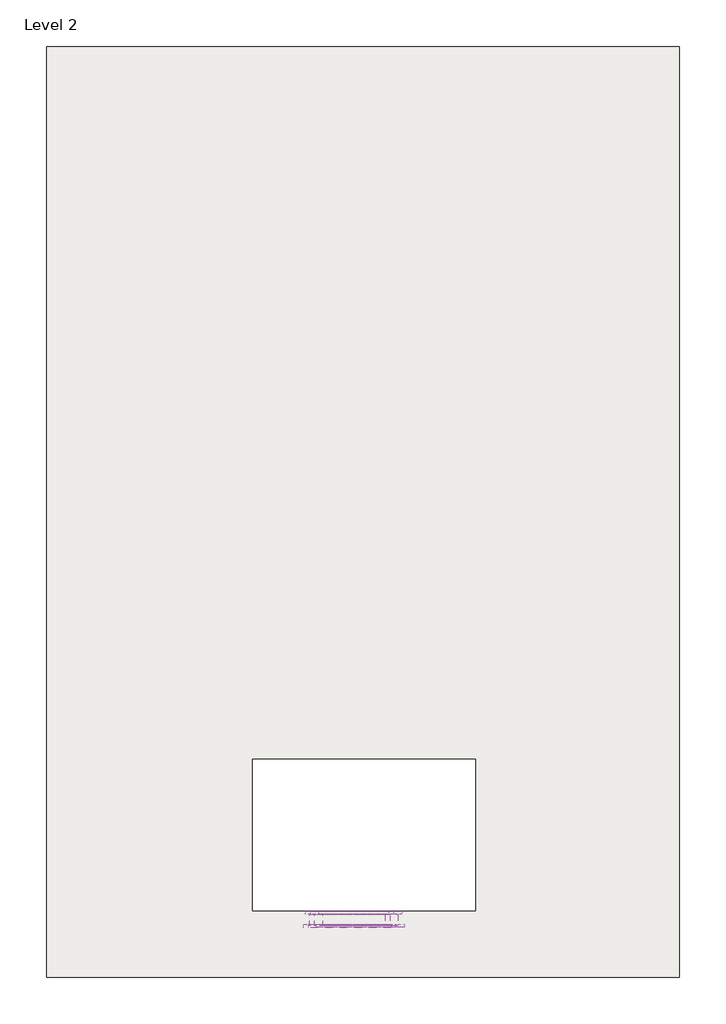
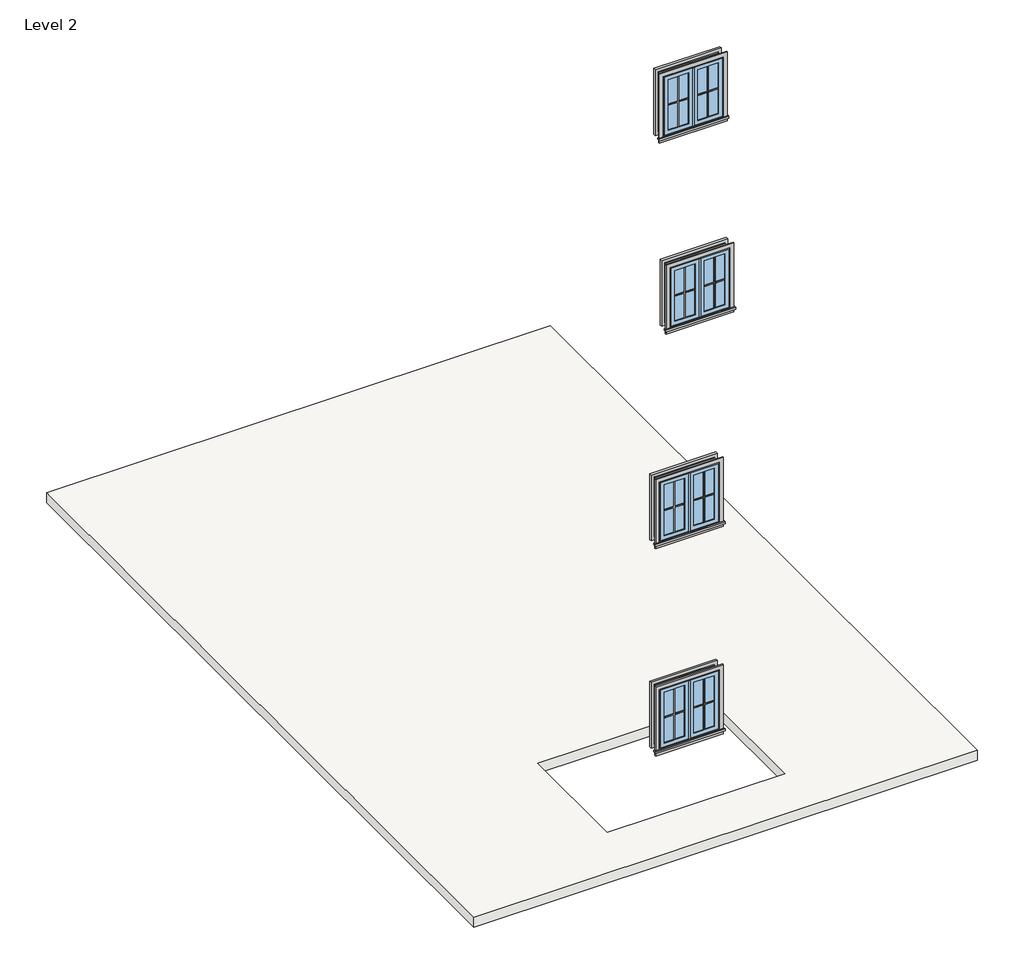
# One storey, incomplete: 16 proxies, 4 windows, 1 roof.
"""IFC4 building model written with IfcOpenShell, lengths in millimetres."""

from ifc_helpers import new_model, si_unit, frame, origin, place, context, project, spatial, polyline, outline, extrude, transform, mapped, element, save
from components import muntin_pattern_2x2_muntin_pattern_2x2_b3fe6957, muntin_pattern_2x2_muntin_pattern_2x2_3e0ecaf2, trim_window_exterior_flat_with_sill_41619996, trim_window_interior_flat_picture_frame_51c85655, window_a598f463

model = new_model("IFC4")

# Units and contexts
model_context = context("Model", 3, world=origin())
ifc_project = project(units=[si_unit("LENGTHUNIT", "METRE", prefix="MILLI")], contexts=[model_context])

# Site, building, storey
site = spatial("IfcSite", under=ifc_project)
building = spatial("IfcBuilding", under=site)
storey = spatial("IfcBuildingStorey", under=building, Name="Level 2", Elevation=3048.0)

# Proxies
placement = place(None, origin())
muntin_pattern_2x2_muntin_pattern_2x2_shape = muntin_pattern_2x2_muntin_pattern_2x2_b3fe6957(model_context)
element("IfcBuildingElementProxy", 1, Name="Muntin Pattern_2x2 : Muntin Pattern_2x2", ObjectType="Muntin Pattern_2x2 : Muntin Pattern_2x2", at=placement, inside=storey, context=model_context, shape_type="MappedRepresentation", body=[
    mapped(muntin_pattern_2x2_muntin_pattern_2x2_shape, transform((-1374.3964614, -4419.8859248, 4410.0195631), x_axis=(-1.0, 0.0, 0.0), y_axis=(0.0, -1.0, 0.0), z_axis=(0.0, 0.0, 1.0))),
])
element("IfcBuildingElementProxy", 2, Name="Muntin Pattern_2x2 : Muntin Pattern_2x2", ObjectType="Muntin Pattern_2x2 : Muntin Pattern_2x2", at=placement, inside=storey, context=model_context, shape_type="MappedRepresentation", body=[
    mapped(muntin_pattern_2x2_muntin_pattern_2x2_shape, transform((-1374.3964614, -4419.8859248, 7567.8197748), x_axis=(-1.0, 0.0, 0.0), y_axis=(0.0, -1.0, 0.0), z_axis=(0.0, 0.0, 1.0))),
])
element("IfcBuildingElementProxy", 3, Name="Muntin Pattern_2x2 : Muntin Pattern_2x2", ObjectType="Muntin Pattern_2x2 : Muntin Pattern_2x2", at=placement, inside=storey, context=model_context, shape_type="MappedRepresentation", body=[
    mapped(muntin_pattern_2x2_muntin_pattern_2x2_shape, transform((-1221.9964614, -4419.8859248, 10781.9890194), x_axis=(-1.0, 0.0, 0.0), y_axis=(0.0, -1.0, 0.0), z_axis=(0.0, 0.0, 1.0))),
])
element("IfcBuildingElementProxy", 4, Name="Muntin Pattern_2x2 : Muntin Pattern_2x2", ObjectType="Muntin Pattern_2x2 : Muntin Pattern_2x2", at=placement, inside=storey, context=model_context, shape_type="MappedRepresentation", body=[
    mapped(muntin_pattern_2x2_muntin_pattern_2x2_shape, transform((-1317.2464614, -4419.8859248, 13724.8067311), x_axis=(-1.0, 0.0, 0.0), y_axis=(0.0, -1.0, 0.0), z_axis=(0.0, 0.0, 1.0))),
])
muntin_pattern_2x2_muntin_pattern_2x2_2_shape = muntin_pattern_2x2_muntin_pattern_2x2_3e0ecaf2(model_context)
element("IfcBuildingElementProxy", 5, Name="Muntin Pattern_2x2 : Muntin Pattern_2x2", ObjectType="Muntin Pattern_2x2 : Muntin Pattern_2x2", at=placement, inside=storey, context=model_context, shape_type="MappedRepresentation", body=[
    mapped(muntin_pattern_2x2_muntin_pattern_2x2_2_shape, transform((-1803.0214614, -4419.8859248, 4410.0195631), x_axis=(1.0, 0.0, 0.0), y_axis=(0.0, 1.0, 0.0), z_axis=(0.0, 0.0, 1.0))),
])
element("IfcBuildingElementProxy", 6, Name="Muntin Pattern_2x2 : Muntin Pattern_2x2", ObjectType="Muntin Pattern_2x2 : Muntin Pattern_2x2", at=placement, inside=storey, context=model_context, shape_type="MappedRepresentation", body=[
    mapped(muntin_pattern_2x2_muntin_pattern_2x2_2_shape, transform((-1803.0214614, -4419.8859248, 7567.8197748), x_axis=(1.0, 0.0, 0.0), y_axis=(0.0, 1.0, 0.0), z_axis=(0.0, 0.0, 1.0))),
])
element("IfcBuildingElementProxy", 7, Name="Muntin Pattern_2x2 : Muntin Pattern_2x2", ObjectType="Muntin Pattern_2x2 : Muntin Pattern_2x2", at=placement, inside=storey, context=model_context, shape_type="MappedRepresentation", body=[
    mapped(muntin_pattern_2x2_muntin_pattern_2x2_2_shape, transform((-1650.6214614, -4419.8859248, 10781.9890194), x_axis=(1.0, 0.0, 0.0), y_axis=(0.0, 1.0, 0.0), z_axis=(0.0, 0.0, 1.0))),
])
element("IfcBuildingElementProxy", 8, Name="Muntin Pattern_2x2 : Muntin Pattern_2x2", ObjectType="Muntin Pattern_2x2 : Muntin Pattern_2x2", at=placement, inside=storey, context=model_context, shape_type="MappedRepresentation", body=[
    mapped(muntin_pattern_2x2_muntin_pattern_2x2_2_shape, transform((-1745.8714614, -4419.8859248, 13724.8067311), x_axis=(1.0, 0.0, 0.0), y_axis=(0.0, 1.0, 0.0), z_axis=(0.0, 0.0, 1.0))),
])
trim_window_exterior_flat_with_sill_shape = trim_window_exterior_flat_with_sill_41619996(model_context)
element("IfcBuildingElementProxy", 9, Name="Trim-Window-Exterior-Flat : with Sill", ObjectType="Trim-Window-Exterior-Flat : with Sill", at=placement, inside=storey, context=model_context, shape_type="MappedRepresentation", body=[
    mapped(trim_window_exterior_flat_with_sill_shape, transform((-1588.7089614, -4429.4109248, 5254.5695631), x_axis=(1.0, 0.0, 0.0), y_axis=(0.0, 0.0, 1.0), z_axis=(0.0, -1.0, 0.0))),
])
element("IfcBuildingElementProxy", 10, Name="Trim-Window-Exterior-Flat : with Sill", ObjectType="Trim-Window-Exterior-Flat : with Sill", at=placement, inside=storey, context=model_context, shape_type="MappedRepresentation", body=[
    mapped(trim_window_exterior_flat_with_sill_shape, transform((-1588.7089614, -4429.4109248, 8412.3697748), x_axis=(1.0, 0.0, 0.0), y_axis=(0.0, 0.0, 1.0), z_axis=(0.0, -1.0, 0.0))),
])
element("IfcBuildingElementProxy", 11, Name="Trim-Window-Exterior-Flat : with Sill", ObjectType="Trim-Window-Exterior-Flat : with Sill", at=placement, inside=storey, context=model_context, shape_type="MappedRepresentation", body=[
    mapped(trim_window_exterior_flat_with_sill_shape, transform((-1436.3089614, -4429.4109248, 11626.5390194), x_axis=(1.0, 0.0, 0.0), y_axis=(0.0, 0.0, 1.0), z_axis=(0.0, -1.0, 0.0))),
])
element("IfcBuildingElementProxy", 12, Name="Trim-Window-Exterior-Flat : with Sill", ObjectType="Trim-Window-Exterior-Flat : with Sill", at=placement, inside=storey, context=model_context, shape_type="MappedRepresentation", body=[
    mapped(trim_window_exterior_flat_with_sill_shape, transform((-1531.5589614, -4429.4109248, 14569.3567311), x_axis=(1.0, 0.0, 0.0), y_axis=(0.0, 0.0, 1.0), z_axis=(0.0, -1.0, 0.0))),
])
trim_window_interior_flat_picture_frame_shape = trim_window_interior_flat_picture_frame_51c85655(model_context)
element("IfcBuildingElementProxy", 13, Name="Trim-Window-Interior-Flat : Picture Frame", ObjectType="Trim-Window-Interior-Flat : Picture Frame", at=placement, inside=storey, context=model_context, shape_type="MappedRepresentation", body=[
    mapped(trim_window_interior_flat_picture_frame_shape, transform((-1588.7089614, -4315.1109248, 5254.5695631), x_axis=(-1.0, 0.0, 0.0), y_axis=(0.0, 0.0, 1.0), z_axis=(0.0, 1.0, 0.0))),
])
element("IfcBuildingElementProxy", 14, Name="Trim-Window-Interior-Flat : Picture Frame", ObjectType="Trim-Window-Interior-Flat : Picture Frame", at=placement, inside=storey, context=model_context, shape_type="MappedRepresentation", body=[
    mapped(trim_window_interior_flat_picture_frame_shape, transform((-1588.7089614, -4315.1109248, 8412.3697748), x_axis=(-1.0, 0.0, 0.0), y_axis=(0.0, 0.0, 1.0), z_axis=(0.0, 1.0, 0.0))),
])
element("IfcBuildingElementProxy", 15, Name="Trim-Window-Interior-Flat : Picture Frame", ObjectType="Trim-Window-Interior-Flat : Picture Frame", at=placement, inside=storey, context=model_context, shape_type="MappedRepresentation", body=[
    mapped(trim_window_interior_flat_picture_frame_shape, transform((-1436.3089614, -4315.1109248, 11626.5390194), x_axis=(-1.0, 0.0, 0.0), y_axis=(0.0, 0.0, 1.0), z_axis=(0.0, 1.0, 0.0))),
])
element("IfcBuildingElementProxy", 16, Name="Trim-Window-Interior-Flat : Picture Frame", ObjectType="Trim-Window-Interior-Flat : Picture Frame", at=placement, inside=storey, context=model_context, shape_type="MappedRepresentation", body=[
    mapped(trim_window_interior_flat_picture_frame_shape, transform((-1531.5589614, -4315.1109248, 14569.3567311), x_axis=(-1.0, 0.0, 0.0), y_axis=(0.0, 0.0, 1.0), z_axis=(0.0, 1.0, 0.0))),
])

# Roof
element("IfcRoof", 17, ObjectType="Generic - 12\"", at=placement, inside=storey, context=model_context, shape_type="SweptSolid", body=[
    extrude(outline(polyline([(2221.2910386, -5039.0109248), (-5036.7589614, -5039.0109248), (-5036.7589614, 5628.9890752), (2221.2910386, 5628.9890752), (2221.2910386, -5039.0109248)]), holes=[polyline([(-116.1777511, -2539.253904), (-2673.8853157, -2539.253904), (-2673.8853157, -4276.2080688), (-116.1777511, -4276.2080688), (-116.1777511, -2539.253904)])]), frame((0.0, 0.0, 3048.0), z_axis=(0.0, 0.0, 1.0), x_axis=(1.0, 0.0, 0.0)), (0.0, 0.0, 1.0), 152.4),
])

# Windows
window_shape = window_a598f463(model_context)
element("IfcWindow", 18, ObjectType="Window-Casement-Double : 34\" x 36\"", at=placement, inside=storey, context=model_context, shape_type="MappedRepresentation", body=[
    mapped(window_shape, transform((-1588.7089614, -4372.2609248, 3425.7695631), x_axis=(-1.0, 0.0, 0.0), y_axis=(0.0, -1.0, 0.0), z_axis=(0.0, 0.0, 1.0))),
])
element("IfcWindow", 19, ObjectType="Window-Casement-Double : 34\" x 36\"", at=placement, inside=storey, context=model_context, shape_type="MappedRepresentation", body=[
    mapped(window_shape, transform((-1588.7089614, -4372.2609248, 6583.5697748), x_axis=(-1.0, 0.0, 0.0), y_axis=(0.0, -1.0, 0.0), z_axis=(0.0, 0.0, 1.0))),
])
element("IfcWindow", 20, ObjectType="Window-Casement-Double : 34\" x 36\"", at=placement, inside=storey, context=model_context, shape_type="MappedRepresentation", body=[
    mapped(window_shape, transform((-1436.3089614, -4372.2609248, 9797.7390194), x_axis=(-1.0, 0.0, 0.0), y_axis=(0.0, -1.0, 0.0), z_axis=(0.0, 0.0, 1.0))),
])
element("IfcWindow", 21, ObjectType="Window-Casement-Double : 34\" x 36\"", at=placement, inside=storey, context=model_context, shape_type="MappedRepresentation", body=[
    mapped(window_shape, transform((-1531.5589614, -4372.2609248, 12740.5567311), x_axis=(-1.0, 0.0, 0.0), y_axis=(0.0, -1.0, 0.0), z_axis=(0.0, 0.0, 1.0))),
])

save(model, "model.ifc")

# Revit data of these elements
# Type "Muntin Pattern_2x2 : Muntin Pattern_2x2"
#   Width [instance default] = 4' - 0"
#   Thickness = 0' - 0 1/2"
#   Height [instance default] = 4' - 0"
#   Distance = 0' - 0 3/4"
#   Interior Material [instance default] = none
#   Exterior Material [instance default] = none
#   Default Elevation = 0
# Type "Trim-Window-Exterior-Flat : with Sill"
#   Trim Width = 0' - 2 1/4"
#   Trim Thickness_Picture Frame = 0' - 1 1/4"
#   Trim Thickness_with Sill = 0' - 0 3/4"
#   Sill Thickness = 0' - 1 1/4"
#   Opening Width [instance default] = 2' - 0"
#   Opening Height [instance default] = 3' - 0"
#   Default Elevation = 4' - 0"
#   Sill = yes
#   Picture Frame = no
#   Trim Material [instance default] = none
# Type "Trim-Window-Interior-Flat : Picture Frame"
#   Trim Thickness_Picture Frame = 0' - 1 1/4"
#   Trim Width = 0' - 2 1/4"
#   Trim Thickness_with Sill = 0' - 0 3/4"
#   Sill Thickness = 0' - 1 1/4"
#   Opening Width [instance default] = 2' - 0"
#   Opening Height [instance default] = 3' - 0"
#   Default Elevation = 4' - 0"
#   Sill = no
#   Picture Frame = yes
#   Trim Material [instance default] = none
# Type "Generic - 12\""
#   Assembly Code = "B1020"
#   Layers, outside or top first: 0' - 6" no material (function 1)
# Type "Window-Casement-Double : 34\" x 36\""
#   Type Mark = "14"
#   Fire Rating = "0.5h"
#   Assembly Code = "B2020100"
#   Analytic Construction = "Double glazing - domestic"
#   Frame Extension [instance default] = 0' - 0 1/4"
#   Window Inset [instance default] = 0' - 0"
#   Wall Thickness [instance default] = 0' - 6"
#   Interior Wall Closure [instance default] = 0' - 2 1/4"
#   Half Width = 1' - 5"
#   Visual Light Transmittance = 0.81
#   Thermal Resistance (R) = 1.8146 (h·ft²·°F)/BTU
#   Solar Heat Gain Coefficient = 0.76
#   Rough Width = 2' - 10 1/2"
#   Rough Height = 3' - 0 1/2"
#   Height = 3' - 0"
#   Heat Transfer Coefficient (U) = 0.5511 BTU/(h·ft²·°F)
#   Exterior Wall Closure [instance default] = 0' - 1 1/4"
#   Extension Jamb [instance default] = 0' - 2 1/4"
#   Default Sill Height = 3' - 0"
#   Width = 2' - 10"
#   Define Thermal Properties by = 0
#   Muntin Visibility = yes
#   Interior Trim Visibility [instance default] = yes
#   Exterior Trim Visibility [instance default] = yes
#   Extension Jamb Visibility [instance default] = yes
#   Interior Trim Material = Wood - Stained
#   Muntin Pattern = Muntin Pattern_2x2 : Muntin Pattern_2x2
#   Interior Trim = Trim-Window-Interior-Flat : Picture Frame
#   Interior Frame Material = Wood - Stained
#   Glass Panel Material = Glass
#   Exterior Trim Material = Clad - White
#   Exterior Trim = Trim-Window-Exterior-Flat : with Sill
#   Exterior Frame Material = Clad - White
#   Wall Closure = (empty or 0)
# Elements 1, 2, 3, 4, 5, 6, 7, 8 (IfcBuildingElementProxy, "Muntin Pattern_2x2 : Muntin Pattern_2x2")
#   Width = 0' - 11 5/8"
#   Height = 2' - 6 1/2"
#   Interior Material = Wood - Stained
#   Exterior Material = Clad - White
#   Phase Created = New Construction
#   Materials on its faces: "Clad - White", "Wood - Stained"
# Elements 9, 10, 11, 12 (IfcBuildingElementProxy, "Trim-Window-Exterior-Flat : with Sill")
#   Opening Width = 2' - 10"
#   Opening Height = 3' - 0"
#   Trim Material = Clad - White
#   Phase Created = New Construction
#   Materials on its faces: "Clad - White"
# Elements 13, 14, 15, 16 (IfcBuildingElementProxy, "Trim-Window-Interior-Flat : Picture Frame")
#   Opening Width = 2' - 10"
#   Opening Height = 3' - 0"
#   Trim Material = Wood - Stained
#   Phase Created = New Construction
#   Materials on its faces: "Wood - Stained"
# Element 17 (IfcRoof, "Generic - 12\"")
#   built-in parameter 1001705 = 10.5 (stored number, unit not read)
#   built-in parameter 1001710 = 33615
#   Phase Created = New Construction
#   Materials on its faces: "Default Roof", "Door - Frame"
# Element 18 (IfcWindow, "Window-Casement-Double : 34\" x 36\"")
#   Mark = "2"
#   Window Inset = 0' - 0"
#   Interior Wall Closure = 0' - 2 1/4"
#   Frame Extension = 0' - 0 1/4"
#   Exterior Wall Closure = 0' - 1 1/4"
#   Interior Trim Visibility = yes
#   Exterior Trim Visibility = yes
#   Phase Created = New Construction
#   Materials on its faces: "Wood - Stained", "Glass", "Clad - White"
# Element 19 (IfcWindow, "Window-Casement-Double : 34\" x 36\"")
#   Mark = "3"
#   Window Inset = 0' - 0"
#   Interior Wall Closure = 0' - 2 1/4"
#   Frame Extension = 0' - 0 1/4"
#   Exterior Wall Closure = 0' - 1 1/4"
#   Interior Trim Visibility = yes
#   Exterior Trim Visibility = yes
#   Phase Created = New Construction
#   Materials on its faces: "Wood - Stained", "Glass", "Clad - White"
# Element 20 (IfcWindow, "Window-Casement-Double : 34\" x 36\"")
#   Mark = "4"
#   Window Inset = 0' - 0"
#   Interior Wall Closure = 0' - 2 1/4"
#   Frame Extension = 0' - 0 1/4"
#   Exterior Wall Closure = 0' - 1 1/4"
#   Interior Trim Visibility = yes
#   Exterior Trim Visibility = yes
#   Phase Created = New Construction
#   Materials on its faces: "Wood - Stained", "Glass", "Clad - White"
# Element 21 (IfcWindow, "Window-Casement-Double : 34\" x 36\"")
#   Mark = "5"
#   Window Inset = 0' - 0"
#   Interior Wall Closure = 0' - 2 1/4"
#   Frame Extension = 0' - 0 1/4"
#   Exterior Wall Closure = 0' - 1 1/4"
#   Interior Trim Visibility = yes
#   Exterior Trim Visibility = yes
#   Phase Created = New Construction
#   Materials on its faces: "Wood - Stained", "Glass", "Clad - White"
# Materials
#   "Wood - Stained": class "Wood", colour RGB 224 178 126, transparency 0, Cost = 0
#   "Glass": class "Glass", colour RGB 0 128 192, transparency 0.75, Description = "Soda Lime Glass", Cost = 0
#   "Clad - White": class "Wood", colour RGB 242 242 238, transparency 0, Cost = 0
#   "Default Roof": colour RGB 88 101 114, transparency 0, Cost = 0
#   "Door - Frame": colour RGB 118 70 51, transparency 0, Cost = 0
